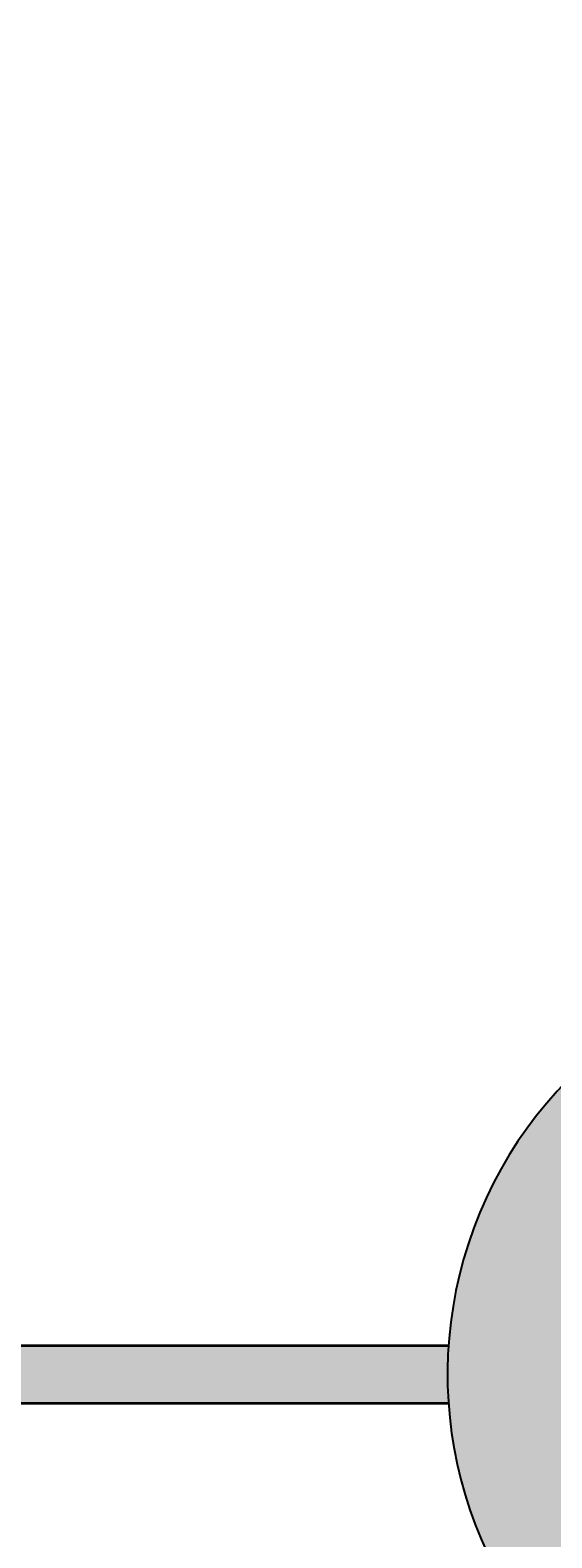
# Model space of a CAD drawing. Units: millimetres. Extents: x -22994 to 29398, y -19990 to 20176.
# Tile 11 of 135: x 32 to 41, y 26 to 52. Entities that reach past the tile are written whole.
import ezdxf
from ezdxf import colors
from ezdxf.entities.mleader import LeaderData, LeaderLine
from ezdxf.math import Vec2, Vec3

# ---------------------------------------------------------------- set-up
doc = ezdxf.new("R2010")
doc.units = ezdxf.units.MM
doc.header["$MEASUREMENT"] = 0
for name, color, linetype, lineweight in [('M-ANNO-TEXT', 7, 'Continuous', 25), ('M-DIMS', 2, 'Continuous', 18), ('M-EQPM', 7, 'Continuous', 25), ('M-EQPM-PATT', 7, 'Continuous', 18), ('M-PIPE', 7, 'Continuous', 35)]:
    doc.layers.add(name, color=color, linetype=linetype, lineweight=lineweight)
doc.styles.get("Standard").update_dxf_attribs({"font": 'arial.ttf'})
doc.dimstyles.get("Standard").update_dxf_attribs({"dimtxt": 0.18, "dimasz": 10000, "dimexe": 0.18, "dimexo": 0.0625, "dimgap": 0.09, "dimtad": 0, "dimtih": 1, "dimtoh": 1, "dimdec": 0, "dimzin": 0, "dimdsep": 46, "dimtxsty": 'Standard', "dimcen": 0.09, "dimadec": 0, "dimazin": 0, "dimtfac": 1, "dimtdec": 0, "dimtofl": 0, "dimtmove": 0, "dimatfit": 3, "dimfxl": 1, "dimtolj": 1, "dimtzin": 0, "dimlwd": 30, "dimarcsym": 0})

# ---------------------------------------------------------------- blocks, each defined once
blk = doc.blocks.new('*D2')
at = {"layer": 'Defpoints', "color": 0, "transparency": 16777216}
for p in [(6.677, 10.271), (290.852, 10.271), (290.852, -5.079)]:
    blk.add_point(p, dxfattribs=at)
at = {"layer": 'M-DIMS', "color": 0, "lineweight": -2, "transparency": 16777216}
for p, q in [((6.677, 10.209), (6.677, -5.259)), ((290.852, 10.209), (290.852, -5.259))]:
    blk.add_line(p, q, dxfattribs=at)
at = {"layer": 'M-DIMS', "color": 0, "lineweight": 30, "transparency": 16777216}
for p, q in [((-9993.323, -5.079), (-19993.323, -5.079)), ((10290.852, -5.079), (20290.852, -5.079))]:
    blk.add_line(p, q, dxfattribs=at)
at = {"layer": 'M-DIMS', "color": 0, "transparency": 16777216}
for points in [[(-9993.323, 1661.588), (-9993.323, -1671.745), (6.677, -5.079)], [(10290.852, 1661.588), (10290.852, -1671.745), (290.852, -5.079)]]:
    blk.add_solid(points, dxfattribs=at)
at = {"layer": 'M-DIMS', "color": 0, "transparency": 16777216, "insert": (148.765, -5.079), "char_height": 0.18, "attachment_point": 5}
blk.add_mtext('\\A1;284.2', dxfattribs=at)
blk = doc.blocks.new('*D3')
at = {"layer": 'Defpoints', "color": 0, "transparency": 16777216}
for p in [(110.265, 204.165), (110.265, 176.366), (95.833, 127.967)]:
    blk.add_point(p, dxfattribs=at)
at = {"layer": 'M-DIMS', "color": 0, "lineweight": -2, "transparency": 16777216}
for p, q in [((95.833, 128.03), (95.833, 204.345)), ((110.265, 176.429), (110.265, 204.345))]:
    blk.add_line(p, q, dxfattribs=at)
at = {"layer": 'M-DIMS', "color": 0, "lineweight": 30, "transparency": 16777216}
for p, q in [((-9904.167, 204.165), (-19904.167, 204.165)), ((10110.265, 204.165), (20110.265, 204.165))]:
    blk.add_line(p, q, dxfattribs=at)
at = {"layer": 'M-DIMS', "color": 0, "transparency": 16777216}
for points in [[(-9904.167, 1870.832), (-9904.167, -1462.501), (95.833, 204.165)], [(10110.265, 1870.832), (10110.265, -1462.501), (110.265, 204.165)]]:
    blk.add_solid(points, dxfattribs=at)
at = {"layer": 'M-DIMS', "color": 0, "transparency": 16777216, "insert": (103.049, 204.165), "char_height": 0.18, "attachment_point": 5}
blk.add_mtext('\\A1;14.432', dxfattribs=at)
blk = doc.blocks.new('*D4')
at = {"layer": 'Defpoints', "color": 0, "transparency": 16777216}
for p in [(116.265, 204.165), (110.265, 176.366), (116.265, 176.366)]:
    blk.add_point(p, dxfattribs=at)
at = {"layer": 'M-DIMS', "color": 0, "lineweight": -2, "transparency": 16777216}
for p, q in [((110.265, 176.429), (110.265, 204.345)), ((116.265, 176.429), (116.265, 204.345))]:
    blk.add_line(p, q, dxfattribs=at)
at = {"layer": 'M-DIMS', "color": 0, "lineweight": 30, "transparency": 16777216}
for p, q in [((-9889.735, 204.165), (-19889.735, 204.165)), ((10116.265, 204.165), (20116.265, 204.165))]:
    blk.add_line(p, q, dxfattribs=at)
at = {"layer": 'M-DIMS', "color": 0, "transparency": 16777216}
for points in [[(-9889.735, 1870.832), (-9889.735, -1462.501), (110.265, 204.165)], [(10116.265, 1870.832), (10116.265, -1462.501), (116.265, 204.165)]]:
    blk.add_solid(points, dxfattribs=at)
at = {"layer": 'M-DIMS', "color": 0, "transparency": 16777216, "insert": (113.265, 204.165), "char_height": 0.18, "attachment_point": 5}
blk.add_mtext('\\A1;6', dxfattribs=at)
blk = doc.blocks.new('*D5')
at = {"layer": 'Defpoints', "color": 0, "transparency": 16777216}
for p in [(181.265, 204.165), (116.265, 176.366), (181.265, 176.366)]:
    blk.add_point(p, dxfattribs=at)
at = {"layer": 'M-DIMS', "color": 0, "lineweight": -2, "transparency": 16777216}
for p, q in [((116.265, 176.429), (116.265, 204.345)), ((181.265, 176.429), (181.265, 204.345))]:
    blk.add_line(p, q, dxfattribs=at)
at = {"layer": 'M-DIMS', "color": 0, "lineweight": 30, "transparency": 16777216}
for p, q in [((-9883.735, 204.165), (-19883.735, 204.165)), ((10181.265, 204.165), (20181.265, 204.165))]:
    blk.add_line(p, q, dxfattribs=at)
at = {"layer": 'M-DIMS', "color": 0, "transparency": 16777216}
for points in [[(-9883.735, 1870.832), (-9883.735, -1462.501), (116.265, 204.165)], [(10181.265, 1870.832), (10181.265, -1462.501), (181.265, 204.165)]]:
    blk.add_solid(points, dxfattribs=at)
at = {"layer": 'M-DIMS', "color": 0, "transparency": 16777216, "insert": (148.765, 204.165), "char_height": 0.18, "attachment_point": 5}
blk.add_mtext('\\A1;65', dxfattribs=at)
blk = doc.blocks.new('*D6')
at = {"layer": 'Defpoints', "color": 0, "transparency": 16777216}
for p in [(187.265, 204.165), (181.265, 176.366), (187.265, 176.366)]:
    blk.add_point(p, dxfattribs=at)
at = {"layer": 'M-DIMS', "color": 0, "lineweight": -2, "transparency": 16777216}
for p, q in [((181.265, 176.429), (181.265, 204.345)), ((187.265, 176.429), (187.265, 204.345))]:
    blk.add_line(p, q, dxfattribs=at)
at = {"layer": 'M-DIMS', "color": 0, "lineweight": 30, "transparency": 16777216}
for p, q in [((-9818.735, 204.165), (-19818.735, 204.165)), ((10187.265, 204.165), (20187.265, 204.165))]:
    blk.add_line(p, q, dxfattribs=at)
at = {"layer": 'M-DIMS', "color": 0, "transparency": 16777216}
for points in [[(-9818.735, 1870.832), (-9818.735, -1462.501), (181.265, 204.165)], [(10187.265, 1870.832), (10187.265, -1462.501), (187.265, 204.165)]]:
    blk.add_solid(points, dxfattribs=at)
at = {"layer": 'M-DIMS', "color": 0, "transparency": 16777216, "insert": (184.265, 204.165), "char_height": 0.18, "attachment_point": 5}
blk.add_mtext('\\A1;6', dxfattribs=at)
blk = doc.blocks.new('*D7')
at = {"layer": 'Defpoints', "color": 0, "transparency": 16777216}
for p in [(201.697, 204.165), (187.265, 176.366), (201.697, 127.967)]:
    blk.add_point(p, dxfattribs=at)
at = {"layer": 'M-DIMS', "color": 0, "lineweight": -2, "transparency": 16777216}
for p, q in [((187.265, 176.429), (187.265, 204.345)), ((201.697, 128.03), (201.697, 204.345))]:
    blk.add_line(p, q, dxfattribs=at)
at = {"layer": 'M-DIMS', "color": 0, "lineweight": 30, "transparency": 16777216}
for p, q in [((-9812.735, 204.165), (-19812.735, 204.165)), ((10201.697, 204.165), (20201.697, 204.165))]:
    blk.add_line(p, q, dxfattribs=at)
at = {"layer": 'M-DIMS', "color": 0, "transparency": 16777216}
for points in [[(-9812.735, 1870.832), (-9812.735, -1462.501), (187.265, 204.165)], [(10201.697, 1870.832), (10201.697, -1462.501), (201.697, 204.165)]]:
    blk.add_solid(points, dxfattribs=at)
at = {"layer": 'M-DIMS', "color": 0, "transparency": 16777216, "insert": (194.481, 204.165), "char_height": 0.18, "attachment_point": 5}
blk.add_mtext('\\A1;14.432', dxfattribs=at)
blk = doc.blocks.new('*D8')
at = {"layer": 'Defpoints', "color": 0, "transparency": 16777216}
for p in [(227.648, 204.165), (227.648, 146.73), (201.697, 127.967)]:
    blk.add_point(p, dxfattribs=at)
at = {"layer": 'M-DIMS', "color": 0, "lineweight": -2, "transparency": 16777216}
for p, q in [((201.697, 128.03), (201.697, 204.345)), ((227.648, 146.792), (227.648, 204.345))]:
    blk.add_line(p, q, dxfattribs=at)
at = {"layer": 'M-DIMS', "color": 0, "lineweight": 30, "transparency": 16777216}
for p, q in [((-9798.303, 204.165), (-19798.303, 204.165)), ((10227.648, 204.165), (20227.648, 204.165))]:
    blk.add_line(p, q, dxfattribs=at)
at = {"layer": 'M-DIMS', "color": 0, "transparency": 16777216}
for points in [[(-9798.303, 1870.832), (-9798.303, -1462.501), (201.697, 204.165)], [(10227.648, 1870.832), (10227.648, -1462.501), (227.648, 204.165)]]:
    blk.add_solid(points, dxfattribs=at)
at = {"layer": 'M-DIMS', "color": 0, "transparency": 16777216, "insert": (214.673, 204.165), "char_height": 0.18, "attachment_point": 5}
blk.add_mtext('\\A1;25.95', dxfattribs=at)
blk = doc.blocks.new('*D9')
at = {"layer": 'Defpoints', "color": 0, "transparency": 16777216}
for p in [(187.265, 176.366), (306.202, 176.366), (290.852, 10.271)]:
    blk.add_point(p, dxfattribs=at)
at = {"layer": 'M-DIMS', "color": 0, "lineweight": 30, "transparency": 16777216}
for p, q in [((306.202, 10176.366), (306.202, 20176.366)), ((306.202, -9989.729), (306.202, -19989.729))]:
    blk.add_line(p, q, dxfattribs=at)
at = {"layer": 'M-DIMS', "color": 0, "lineweight": -2, "transparency": 16777216}
for p, q in [((187.327, 176.366), (306.382, 176.366)), ((290.915, 10.271), (306.382, 10.271))]:
    blk.add_line(p, q, dxfattribs=at)
at = {"layer": 'M-DIMS', "color": 0, "transparency": 16777216}
for points in [[(-1360.465, 10176.366), (1972.869, 10176.366), (306.202, 176.366)], [(-1360.465, -9989.729), (1972.869, -9989.729), (306.202, 10.271)]]:
    blk.add_solid(points, dxfattribs=at)
at = {"layer": 'M-DIMS', "color": 0, "transparency": 16777216, "insert": (306.202, 93.319), "char_height": 0.18, "attachment_point": 5}
blk.add_mtext('\\A1;166.1', dxfattribs=at)
blk = doc.blocks.new('*D10')
at = {"layer": 'Defpoints', "color": 0, "transparency": 16777216}
for p in [(125.65, 136.071), (133.346, 136.071), (133.346, -5.079)]:
    blk.add_point(p, dxfattribs=at)
at = {"layer": 'M-DIMS', "color": 0, "lineweight": -2, "transparency": 16777216}
for p, q in [((125.65, 136.009), (125.65, -5.259)), ((133.346, 136.009), (133.346, -5.259))]:
    blk.add_line(p, q, dxfattribs=at)
at = {"layer": 'M-DIMS', "color": 0, "lineweight": 30, "transparency": 16777216}
for p, q in [((-9874.35, -5.079), (-19874.35, -5.079)), ((10133.346, -5.079), (20133.346, -5.079))]:
    blk.add_line(p, q, dxfattribs=at)
at = {"layer": 'M-DIMS', "color": 0, "transparency": 16777216}
for points in [[(-9874.35, 1661.588), (-9874.35, -1671.745), (125.65, -5.079)], [(10133.346, 1661.588), (10133.346, -1671.745), (133.346, -5.079)]]:
    blk.add_solid(points, dxfattribs=at)
at = {"layer": 'M-DIMS', "color": 0, "transparency": 16777216, "insert": (129.498, -5.079), "char_height": 0.18, "attachment_point": 5}
blk.add_mtext('\\A1;7.696', dxfattribs=at)
blk = doc.blocks.new('*D11')
at = {"layer": 'Defpoints', "color": 0, "transparency": 16777216}
for p in [(133.346, 136.071), (135.65, 136.071), (135.65, -5.079)]:
    blk.add_point(p, dxfattribs=at)
at = {"layer": 'M-DIMS', "color": 0, "lineweight": -2, "transparency": 16777216}
for p, q in [((133.346, 136.009), (133.346, -5.259)), ((135.65, 136.009), (135.65, -5.259))]:
    blk.add_line(p, q, dxfattribs=at)
at = {"layer": 'M-DIMS', "color": 0, "lineweight": 30, "transparency": 16777216}
for p, q in [((-9866.654, -5.079), (-19866.654, -5.079)), ((10135.65, -5.079), (20135.65, -5.079))]:
    blk.add_line(p, q, dxfattribs=at)
at = {"layer": 'M-DIMS', "color": 0, "transparency": 16777216}
for points in [[(-9866.654, 1661.588), (-9866.654, -1671.745), (133.346, -5.079)], [(10135.65, 1661.588), (10135.65, -1671.745), (135.65, -5.079)]]:
    blk.add_solid(points, dxfattribs=at)
at = {"layer": 'M-DIMS', "color": 0, "transparency": 16777216, "insert": (134.498, -5.079), "char_height": 0.18, "attachment_point": 5}
blk.add_mtext('\\A1;2.304', dxfattribs=at)
blk = doc.blocks.new('*D12')
at = {"layer": 'Defpoints', "color": 0, "transparency": 16777216}
for p in [(135.65, 136.071), (145.65, 136.071), (145.65, -5.079)]:
    blk.add_point(p, dxfattribs=at)
at = {"layer": 'M-DIMS', "color": 0, "lineweight": -2, "transparency": 16777216}
for p, q in [((135.65, 136.009), (135.65, -5.259)), ((145.65, 136.009), (145.65, -5.259))]:
    blk.add_line(p, q, dxfattribs=at)
at = {"layer": 'M-DIMS', "color": 0, "lineweight": 30, "transparency": 16777216}
for p, q in [((-9864.35, -5.079), (-19864.35, -5.079)), ((10145.65, -5.079), (20145.65, -5.079))]:
    blk.add_line(p, q, dxfattribs=at)
at = {"layer": 'M-DIMS', "color": 0, "transparency": 16777216}
for points in [[(-9864.35, 1661.588), (-9864.35, -1671.745), (135.65, -5.079)], [(10145.65, 1661.588), (10145.65, -1671.745), (145.65, -5.079)]]:
    blk.add_solid(points, dxfattribs=at)
at = {"layer": 'M-DIMS', "color": 0, "transparency": 16777216, "insert": (140.65, -5.079), "char_height": 0.18, "attachment_point": 5}
blk.add_mtext('\\A1;10', dxfattribs=at)
blk = doc.blocks.new('*D13')
at = {"layer": 'Defpoints', "color": 0, "transparency": 16777216}
for p in [(145.65, 136.071), (155.65, 136.071), (155.65, -5.079)]:
    blk.add_point(p, dxfattribs=at)
at = {"layer": 'M-DIMS', "color": 0, "lineweight": -2, "transparency": 16777216}
for p, q in [((145.65, 136.009), (145.65, -5.259)), ((155.65, 136.009), (155.65, -5.259))]:
    blk.add_line(p, q, dxfattribs=at)
at = {"layer": 'M-DIMS', "color": 0, "lineweight": 30, "transparency": 16777216}
for p, q in [((-9854.35, -5.079), (-19854.35, -5.079)), ((10155.65, -5.079), (20155.65, -5.079))]:
    blk.add_line(p, q, dxfattribs=at)
at = {"layer": 'M-DIMS', "color": 0, "transparency": 16777216}
for points in [[(-9854.35, 1661.588), (-9854.35, -1671.745), (145.65, -5.079)], [(10155.65, 1661.588), (10155.65, -1671.745), (155.65, -5.079)]]:
    blk.add_solid(points, dxfattribs=at)
at = {"layer": 'M-DIMS', "color": 0, "transparency": 16777216, "insert": (150.65, -5.079), "char_height": 0.18, "attachment_point": 5}
blk.add_mtext('\\A1;10', dxfattribs=at)
blk = doc.blocks.new('*D14')
at = {"layer": 'Defpoints', "color": 0, "transparency": 16777216}
for p in [(155.65, 136.071), (165.65, 136.071), (165.65, -5.079)]:
    blk.add_point(p, dxfattribs=at)
at = {"layer": 'M-DIMS', "color": 0, "lineweight": -2, "transparency": 16777216}
for p, q in [((155.65, 136.009), (155.65, -5.259)), ((165.65, 136.009), (165.65, -5.259))]:
    blk.add_line(p, q, dxfattribs=at)
at = {"layer": 'M-DIMS', "color": 0, "lineweight": 30, "transparency": 16777216}
for p, q in [((-9844.35, -5.079), (-19844.35, -5.079)), ((10165.65, -5.079), (20165.65, -5.079))]:
    blk.add_line(p, q, dxfattribs=at)
at = {"layer": 'M-DIMS', "color": 0, "transparency": 16777216}
for points in [[(-9844.35, 1661.588), (-9844.35, -1671.745), (155.65, -5.079)], [(10165.65, 1661.588), (10165.65, -1671.745), (165.65, -5.079)]]:
    blk.add_solid(points, dxfattribs=at)
at = {"layer": 'M-DIMS', "color": 0, "transparency": 16777216, "insert": (160.65, -5.079), "char_height": 0.18, "attachment_point": 5}
blk.add_mtext('\\A1;10', dxfattribs=at)
blk = doc.blocks.new('*D15')
at = {"layer": 'Defpoints', "color": 0, "transparency": 16777216}
for p in [(173.346, 154.788), (173.346, 136.071), (306.202, 136.071)]:
    blk.add_point(p, dxfattribs=at)
at = {"layer": 'M-DIMS', "color": 0, "lineweight": 30, "transparency": 16777216}
for p, q in [((306.202, 10154.788), (306.202, 20154.788)), ((306.202, -9863.929), (306.202, -19863.929))]:
    blk.add_line(p, q, dxfattribs=at)
at = {"layer": 'M-DIMS', "color": 0, "lineweight": -2, "transparency": 16777216}
for p, q in [((173.408, 154.788), (306.382, 154.788)), ((173.408, 136.071), (306.382, 136.071))]:
    blk.add_line(p, q, dxfattribs=at)
at = {"layer": 'M-DIMS', "color": 0, "transparency": 16777216}
for points in [[(-1360.465, 10154.788), (1972.869, 10154.788), (306.202, 154.788)], [(-1360.465, -9863.929), (1972.869, -9863.929), (306.202, 136.071)]]:
    blk.add_solid(points, dxfattribs=at)
at = {"layer": 'M-DIMS', "color": 0, "transparency": 16777216, "insert": (306.202, 145.43), "char_height": 0.18, "attachment_point": 5}
blk.add_mtext('\\A1;18.717', dxfattribs=at)
blk = doc.blocks.new('*D16')
at = {"layer": 'Defpoints', "color": 0, "transparency": 16777216}
for p in [(120.17, 204.165), (110.466, 48.035), (120.17, 48.035)]:
    blk.add_point(p, dxfattribs=at)
at = {"layer": 'M-DIMS', "color": 0, "lineweight": -2, "transparency": 16777216}
for p, q in [((110.466, 48.097), (110.466, 204.345)), ((120.17, 48.097), (120.17, 204.345))]:
    blk.add_line(p, q, dxfattribs=at)
at = {"layer": 'M-DIMS', "color": 0, "lineweight": 30, "transparency": 16777216}
for p, q in [((-9889.534, 204.165), (-19889.534, 204.165)), ((10120.17, 204.165), (20120.17, 204.165))]:
    blk.add_line(p, q, dxfattribs=at)
at = {"layer": 'M-DIMS', "color": 0, "transparency": 16777216}
for points in [[(-9889.534, 1870.832), (-9889.534, -1462.501), (110.466, 204.165)], [(10120.17, 1870.832), (10120.17, -1462.501), (120.17, 204.165)]]:
    blk.add_solid(points, dxfattribs=at)
at = {"layer": 'M-DIMS', "color": 0, "transparency": 16777216, "insert": (115.318, 204.165), "char_height": 0.18, "attachment_point": 5}
blk.add_mtext('\\A1;9.704', dxfattribs=at)
blk = doc.blocks.new('*D17')
at = {"layer": 'Defpoints', "color": 0, "transparency": 16777216}
for p in [(126.17, 204.165), (120.17, 48.035), (126.17, 48.035)]:
    blk.add_point(p, dxfattribs=at)
at = {"layer": 'M-DIMS', "color": 0, "lineweight": -2, "transparency": 16777216}
for p, q in [((120.17, 48.097), (120.17, 204.345)), ((126.17, 48.097), (126.17, 204.345))]:
    blk.add_line(p, q, dxfattribs=at)
at = {"layer": 'M-DIMS', "color": 0, "lineweight": 30, "transparency": 16777216}
for p, q in [((-9879.83, 204.165), (-19879.83, 204.165)), ((10126.17, 204.165), (20126.17, 204.165))]:
    blk.add_line(p, q, dxfattribs=at)
at = {"layer": 'M-DIMS', "color": 0, "transparency": 16777216}
for points in [[(-9879.83, 1870.832), (-9879.83, -1462.501), (120.17, 204.165)], [(10126.17, 1870.832), (10126.17, -1462.501), (126.17, 204.165)]]:
    blk.add_solid(points, dxfattribs=at)
at = {"layer": 'M-DIMS', "color": 0, "transparency": 16777216, "insert": (123.17, 204.165), "char_height": 0.18, "attachment_point": 5}
blk.add_mtext('\\A1;6', dxfattribs=at)
blk = doc.blocks.new('*D18')
at = {"layer": 'Defpoints', "color": 0, "transparency": 16777216}
for p in [(132.17, 204.165), (126.17, 48.035), (132.17, 48.035)]:
    blk.add_point(p, dxfattribs=at)
at = {"layer": 'M-DIMS', "color": 0, "lineweight": -2, "transparency": 16777216}
for p, q in [((126.17, 48.097), (126.17, 204.345)), ((132.17, 48.097), (132.17, 204.345))]:
    blk.add_line(p, q, dxfattribs=at)
at = {"layer": 'M-DIMS', "color": 0, "lineweight": 30, "transparency": 16777216}
for p, q in [((-9873.83, 204.165), (-19873.83, 204.165)), ((10132.17, 204.165), (20132.17, 204.165))]:
    blk.add_line(p, q, dxfattribs=at)
at = {"layer": 'M-DIMS', "color": 0, "transparency": 16777216}
for points in [[(-9873.83, 1870.832), (-9873.83, -1462.501), (126.17, 204.165)], [(10132.17, 1870.832), (10132.17, -1462.501), (132.17, 204.165)]]:
    blk.add_solid(points, dxfattribs=at)
at = {"layer": 'M-DIMS', "color": 0, "transparency": 16777216, "insert": (129.17, 204.165), "char_height": 0.18, "attachment_point": 5}
blk.add_mtext('\\A1;6', dxfattribs=at)
blk = doc.blocks.new('*D19')
at = {"layer": 'Defpoints', "color": 0, "transparency": 16777216}
for p in [(138.17, 204.165), (132.17, 48.035), (138.17, 48.035)]:
    blk.add_point(p, dxfattribs=at)
at = {"layer": 'M-DIMS', "color": 0, "lineweight": -2, "transparency": 16777216}
for p, q in [((132.17, 48.097), (132.17, 204.345)), ((138.17, 48.097), (138.17, 204.345))]:
    blk.add_line(p, q, dxfattribs=at)
at = {"layer": 'M-DIMS', "color": 0, "lineweight": 30, "transparency": 16777216}
for p, q in [((-9867.83, 204.165), (-19867.83, 204.165)), ((10138.17, 204.165), (20138.17, 204.165))]:
    blk.add_line(p, q, dxfattribs=at)
at = {"layer": 'M-DIMS', "color": 0, "transparency": 16777216}
for points in [[(-9867.83, 1870.832), (-9867.83, -1462.501), (132.17, 204.165)], [(10138.17, 1870.832), (10138.17, -1462.501), (138.17, 204.165)]]:
    blk.add_solid(points, dxfattribs=at)
at = {"layer": 'M-DIMS', "color": 0, "transparency": 16777216, "insert": (135.17, 204.165), "char_height": 0.18, "attachment_point": 5}
blk.add_mtext('\\A1;6', dxfattribs=at)
blk = doc.blocks.new('*D20')
at = {"layer": 'Defpoints', "color": 0, "transparency": 16777216}
for p in [(144.17, 204.165), (138.17, 48.035), (144.17, 48.035)]:
    blk.add_point(p, dxfattribs=at)
at = {"layer": 'M-DIMS', "color": 0, "lineweight": -2, "transparency": 16777216}
for p, q in [((138.17, 48.097), (138.17, 204.345)), ((144.17, 48.097), (144.17, 204.345))]:
    blk.add_line(p, q, dxfattribs=at)
at = {"layer": 'M-DIMS', "color": 0, "lineweight": 30, "transparency": 16777216}
for p, q in [((-9861.83, 204.165), (-19861.83, 204.165)), ((10144.17, 204.165), (20144.17, 204.165))]:
    blk.add_line(p, q, dxfattribs=at)
at = {"layer": 'M-DIMS', "color": 0, "transparency": 16777216}
for points in [[(-9861.83, 1870.832), (-9861.83, -1462.501), (138.17, 204.165)], [(10144.17, 1870.832), (10144.17, -1462.501), (144.17, 204.165)]]:
    blk.add_solid(points, dxfattribs=at)
at = {"layer": 'M-DIMS', "color": 0, "transparency": 16777216, "insert": (141.17, 204.165), "char_height": 0.18, "attachment_point": 5}
blk.add_mtext('\\A1;6', dxfattribs=at)
blk = doc.blocks.new('*D21')
at = {"layer": 'Defpoints', "color": 0, "transparency": 16777216}
for p in [(149.116, 204.165), (144.17, 48.035), (149.116, 48.035)]:
    blk.add_point(p, dxfattribs=at)
at = {"layer": 'M-DIMS', "color": 0, "lineweight": -2, "transparency": 16777216}
for p, q in [((144.17, 48.097), (144.17, 204.345)), ((149.116, 48.097), (149.116, 204.345))]:
    blk.add_line(p, q, dxfattribs=at)
at = {"layer": 'M-DIMS', "color": 0, "lineweight": 30, "transparency": 16777216}
for p, q in [((-9855.83, 204.165), (-19855.83, 204.165)), ((10149.116, 204.165), (20149.116, 204.165))]:
    blk.add_line(p, q, dxfattribs=at)
at = {"layer": 'M-DIMS', "color": 0, "transparency": 16777216}
for points in [[(-9855.83, 1870.832), (-9855.83, -1462.501), (144.17, 204.165)], [(10149.116, 1870.832), (10149.116, -1462.501), (149.116, 204.165)]]:
    blk.add_solid(points, dxfattribs=at)
at = {"layer": 'M-DIMS', "color": 0, "transparency": 16777216, "insert": (146.643, 204.165), "char_height": 0.18, "attachment_point": 5}
blk.add_mtext('\\A1;4.945', dxfattribs=at)
blk = doc.blocks.new('*D22')
at = {"layer": 'Defpoints', "color": 0, "transparency": 16777216}
for p in [(149.116, 30.99), (155.116, 30.99), (155.116, -5.079)]:
    blk.add_point(p, dxfattribs=at)
at = {"layer": 'M-DIMS', "color": 0, "lineweight": -2, "transparency": 16777216}
for p, q in [((149.116, 30.927), (149.116, -5.259)), ((155.116, 30.927), (155.116, -5.259))]:
    blk.add_line(p, q, dxfattribs=at)
at = {"layer": 'M-DIMS', "color": 0, "lineweight": 30, "transparency": 16777216}
for p, q in [((-9850.884, -5.079), (-19850.884, -5.079)), ((10155.116, -5.079), (20155.116, -5.079))]:
    blk.add_line(p, q, dxfattribs=at)
at = {"layer": 'M-DIMS', "color": 0, "transparency": 16777216}
for points in [[(-9850.884, 1661.588), (-9850.884, -1671.745), (149.116, -5.079)], [(10155.116, 1661.588), (10155.116, -1671.745), (155.116, -5.079)]]:
    blk.add_solid(points, dxfattribs=at)
at = {"layer": 'M-DIMS', "color": 0, "transparency": 16777216, "insert": (152.116, -5.079), "char_height": 0.18, "attachment_point": 5}
blk.add_mtext('\\A1;6', dxfattribs=at)
blk = doc.blocks.new('*D23')
at = {"layer": 'Defpoints', "color": 0, "transparency": 16777216}
for p in [(155.116, 30.99), (161.116, 30.99), (161.116, -5.079)]:
    blk.add_point(p, dxfattribs=at)
at = {"layer": 'M-DIMS', "color": 0, "lineweight": -2, "transparency": 16777216}
for p, q in [((155.116, 30.927), (155.116, -5.259)), ((161.116, 30.927), (161.116, -5.259))]:
    blk.add_line(p, q, dxfattribs=at)
at = {"layer": 'M-DIMS', "color": 0, "lineweight": 30, "transparency": 16777216}
for p, q in [((-9844.884, -5.079), (-19844.884, -5.079)), ((10161.116, -5.079), (20161.116, -5.079))]:
    blk.add_line(p, q, dxfattribs=at)
at = {"layer": 'M-DIMS', "color": 0, "transparency": 16777216}
for points in [[(-9844.884, 1661.588), (-9844.884, -1671.745), (155.116, -5.079)], [(10161.116, 1661.588), (10161.116, -1671.745), (161.116, -5.079)]]:
    blk.add_solid(points, dxfattribs=at)
at = {"layer": 'M-DIMS', "color": 0, "transparency": 16777216, "insert": (158.116, -5.079), "char_height": 0.18, "attachment_point": 5}
blk.add_mtext('\\A1;6', dxfattribs=at)
blk = doc.blocks.new('*D24')
at = {"layer": 'Defpoints', "color": 0, "transparency": 16777216}
for p in [(161.116, 30.99), (166.439, 30.99), (166.439, -5.079)]:
    blk.add_point(p, dxfattribs=at)
at = {"layer": 'M-DIMS', "color": 0, "lineweight": -2, "transparency": 16777216}
for p, q in [((161.116, 30.927), (161.116, -5.259)), ((166.439, 30.927), (166.439, -5.259))]:
    blk.add_line(p, q, dxfattribs=at)
at = {"layer": 'M-DIMS', "color": 0, "lineweight": 30, "transparency": 16777216}
for p, q in [((-9838.884, -5.079), (-19838.884, -5.079)), ((10166.439, -5.079), (20166.439, -5.079))]:
    blk.add_line(p, q, dxfattribs=at)
at = {"layer": 'M-DIMS', "color": 0, "transparency": 16777216}
for points in [[(-9838.884, 1661.588), (-9838.884, -1671.745), (161.116, -5.079)], [(10166.439, 1661.588), (10166.439, -1671.745), (166.439, -5.079)]]:
    blk.add_solid(points, dxfattribs=at)
at = {"layer": 'M-DIMS', "color": 0, "transparency": 16777216, "insert": (163.777, -5.079), "char_height": 0.18, "attachment_point": 5}
blk.add_mtext('\\A1;5.323', dxfattribs=at)
blk = doc.blocks.new('*D25')
at = {"layer": 'Defpoints', "color": 0, "transparency": 16777216}
for p in [(166.439, 30.99), (172.439, 30.99), (172.439, -5.079)]:
    blk.add_point(p, dxfattribs=at)
at = {"layer": 'M-DIMS', "color": 0, "lineweight": -2, "transparency": 16777216}
for p, q in [((166.439, 30.927), (166.439, -5.259)), ((172.439, 30.927), (172.439, -5.259))]:
    blk.add_line(p, q, dxfattribs=at)
at = {"layer": 'M-DIMS', "color": 0, "lineweight": 30, "transparency": 16777216}
for p, q in [((-9833.561, -5.079), (-19833.561, -5.079)), ((10172.439, -5.079), (20172.439, -5.079))]:
    blk.add_line(p, q, dxfattribs=at)
at = {"layer": 'M-DIMS', "color": 0, "transparency": 16777216}
for points in [[(-9833.561, 1661.588), (-9833.561, -1671.745), (166.439, -5.079)], [(10172.439, 1661.588), (10172.439, -1671.745), (172.439, -5.079)]]:
    blk.add_solid(points, dxfattribs=at)
at = {"layer": 'M-DIMS', "color": 0, "transparency": 16777216, "insert": (169.439, -5.079), "char_height": 0.18, "attachment_point": 5}
blk.add_mtext('\\A1;6', dxfattribs=at)
blk = doc.blocks.new('*D26')
at = {"layer": 'Defpoints', "color": 0, "transparency": 16777216}
for p in [(172.439, 30.99), (178.439, 30.99), (178.439, -5.079)]:
    blk.add_point(p, dxfattribs=at)
at = {"layer": 'M-DIMS', "color": 0, "lineweight": -2, "transparency": 16777216}
for p, q in [((172.439, 30.927), (172.439, -5.259)), ((178.439, 30.927), (178.439, -5.259))]:
    blk.add_line(p, q, dxfattribs=at)
at = {"layer": 'M-DIMS', "color": 0, "lineweight": 30, "transparency": 16777216}
for p, q in [((-9827.561, -5.079), (-19827.561, -5.079)), ((10178.439, -5.079), (20178.439, -5.079))]:
    blk.add_line(p, q, dxfattribs=at)
at = {"layer": 'M-DIMS', "color": 0, "transparency": 16777216}
for points in [[(-9827.561, 1661.588), (-9827.561, -1671.745), (172.439, -5.079)], [(10178.439, 1661.588), (10178.439, -1671.745), (178.439, -5.079)]]:
    blk.add_solid(points, dxfattribs=at)
at = {"layer": 'M-DIMS', "color": 0, "transparency": 16777216, "insert": (175.439, -5.079), "char_height": 0.18, "attachment_point": 5}
blk.add_mtext('\\A1;6', dxfattribs=at)
blk = doc.blocks.new('*D27')
at = {"layer": 'Defpoints', "color": 0, "transparency": 16777216}
for p in [(178.439, 30.99), (188.117, 30.99), (188.117, -5.079)]:
    blk.add_point(p, dxfattribs=at)
at = {"layer": 'M-DIMS', "color": 0, "lineweight": -2, "transparency": 16777216}
for p, q in [((178.439, 30.927), (178.439, -5.259)), ((188.117, 30.927), (188.117, -5.259))]:
    blk.add_line(p, q, dxfattribs=at)
at = {"layer": 'M-DIMS', "color": 0, "lineweight": 30, "transparency": 16777216}
for p, q in [((-9821.561, -5.079), (-19821.561, -5.079)), ((10188.117, -5.079), (20188.117, -5.079))]:
    blk.add_line(p, q, dxfattribs=at)
at = {"layer": 'M-DIMS', "color": 0, "transparency": 16777216}
for points in [[(-9821.561, 1661.588), (-9821.561, -1671.745), (178.439, -5.079)], [(10188.117, 1661.588), (10188.117, -1671.745), (188.117, -5.079)]]:
    blk.add_solid(points, dxfattribs=at)
at = {"layer": 'M-DIMS', "color": 0, "transparency": 16777216, "insert": (183.278, -5.079), "char_height": 0.18, "attachment_point": 5}
blk.add_mtext('\\A1;9.679', dxfattribs=at)
blk = doc.blocks.new('*D28')
at = {"layer": 'Defpoints', "color": 0, "transparency": 16777216}
for p in [(188.117, 48.035), (306.202, 48.035), (188.117, 30.99)]:
    blk.add_point(p, dxfattribs=at)
at = {"layer": 'M-DIMS', "color": 0, "lineweight": 30, "transparency": 16777216}
for p, q in [((306.202, 10048.035), (306.202, 20048.035)), ((306.202, -9969.01), (306.202, -19969.01))]:
    blk.add_line(p, q, dxfattribs=at)
at = {"layer": 'M-DIMS', "color": 0, "lineweight": -2, "transparency": 16777216}
for p, q in [((188.18, 48.035), (306.382, 48.035)), ((188.18, 30.99), (306.382, 30.99))]:
    blk.add_line(p, q, dxfattribs=at)
at = {"layer": 'M-DIMS', "color": 0, "transparency": 16777216}
for points in [[(-1360.465, 10048.035), (1972.869, 10048.035), (306.202, 48.035)], [(-1360.465, -9969.01), (1972.869, -9969.01), (306.202, 30.99)]]:
    blk.add_solid(points, dxfattribs=at)
at = {"layer": 'M-DIMS', "color": 0, "transparency": 16777216, "insert": (306.202, 39.512), "char_height": 0.18, "attachment_point": 5}
blk.add_mtext('\\A1;17.045', dxfattribs=at)
blk = doc.blocks.new('*D29')
at = {"layer": 'Defpoints', "color": 0, "transparency": 16777216}
for p in [(36.801, 80.045), (64.03, 80.045)]:
    blk.add_point(p, dxfattribs=at)
at = {"layer": 'M-DIMS', "color": 0, "lineweight": -2, "transparency": 16777216}
for p, q in [((50.415, 79.955), (50.415, 80.135)), ((50.325, 80.045), (50.505, 80.045))]:
    blk.add_line(p, q, dxfattribs=at)
at = {"layer": 'M-DIMS', "color": 0, "lineweight": 30, "transparency": 16777216}
blk.add_line((20064.03, 80.03), (10064.03, 80.038), dxfattribs=at)
at = {"layer": 'M-DIMS', "color": 0, "transparency": 16777216}
blk.add_solid([(10064.031, 1746.704), (10064.028, -1586.629), (64.03, 80.045)], dxfattribs=at)
at = {"layer": 'M-DIMS', "color": 0, "transparency": 16777216, "insert": (20064.521, 80.03), "char_height": 0.18, "attachment_point": 5}
blk.add_mtext('\\A1;∅27.23', dxfattribs=at)
blk = doc.blocks.new('*D32')
at = {"layer": 'Defpoints', "color": 0, "transparency": 16777216}
for p in [(57.164, 118.614), (52.413, 113.093)]:
    blk.add_point(p, dxfattribs=at)
at = {"layer": 'M-DIMS', "color": 0, "lineweight": -2, "transparency": 16777216}
for p, q in [((57.074, 118.614), (57.254, 118.614)), ((57.164, 118.524), (57.164, 118.704))]:
    blk.add_line(p, q, dxfattribs=at)
at = {"layer": 'M-DIMS', "color": 0, "lineweight": 30, "transparency": 16777216}
for p, q in [((-12992.534, -15047.031), (-6470.06, -7466.969)), ((-22992.534, -15047.031), (-12992.534, -15047.031))]:
    blk.add_line(p, q, dxfattribs=at)
at = {"layer": 'M-DIMS', "color": 0, "transparency": 16777216}
blk.add_solid([(-7733.404, -6379.89), (-5206.717, -8554.048), (52.413, 113.093)], dxfattribs=at)
at = {"layer": 'M-DIMS', "color": 0, "transparency": 16777216, "insert": (-22993.208, -15047.031), "char_height": 0.18, "attachment_point": 5}
blk.add_mtext('\\A1;2X R7.284', dxfattribs=at)
blk = doc.blocks.new('*D36')
at = {"layer": 'Defpoints', "color": 0, "transparency": 16777216}
for p in [(46.39, 31.303), (46.387, 26.593)]:
    blk.add_point(p, dxfattribs=at)
at = {"layer": 'M-DIMS', "color": 0, "lineweight": 30, "transparency": 16777216}
for p, q in [((57.15, 20031.301), (51.77, 10031.302)), ((10057.15, 20031.301), (57.15, 20031.301))]:
    blk.add_line(p, q, dxfattribs=at)
at = {"layer": 'M-DIMS', "color": 0, "lineweight": -2, "transparency": 16777216}
for p, q in [((46.389, 28.858), (46.389, 29.038)), ((46.299, 28.948), (46.479, 28.948))]:
    blk.add_line(p, q, dxfattribs=at)
at = {"layer": 'M-DIMS', "color": 0, "transparency": 16777216}
blk.add_solid([(-1614.896, 10032.199), (1718.436, 10030.405), (46.39, 31.303)], dxfattribs=at)
at = {"layer": 'M-DIMS', "color": 0, "transparency": 16777216, "insert": (10057.554, 20031.301), "char_height": 0.18, "attachment_point": 5}
blk.add_mtext('\\A1;∅4.71', dxfattribs=at)

msp = doc.modelspace()

# ---------------------------------------------------------------- hatches: boundary and pattern name
at = {"layer": 'M-EQPM-PATT'}
h = msp.add_hatch(color=256, dxfattribs=at)
h.set_gradient(color1=(242, 103, 34), color2=(242, 103, 34), tint=1, name='CYLINDER')
h.paths.add_polyline_path([(53.5912, 30.0354), (64.8905, 30.0354), (64.8905, 36.2325), (46.3887, 36.2325, 2.6954641)])
h.paths.add_polyline_path([(44.0337, 28.9485, -1), (48.7438, 28.9485, -1)], flags=16)
h.paths.add_polyline_path([(75.6657, 119.7012), (75.6657, 125.8983), (57.1639, 125.8983, 2.6954641), (64.3664, 119.7012)])
h.paths.add_polyline_path([(59.4936, 118.6143, -1), (54.8343, 118.6143, -1)], flags=16)
h = msp.add_hatch(color=256, dxfattribs=at)
h.set_gradient(color1=(16, 86, 137), color2=(39, 118, 187), tint=1, name='CYLINDER')
h.paths.add_polyline_path([(22.8402, 76.5922), (37.2457, 76.5922, -0.0188178), (37.0234, 77.5922), (21.8402, 77.5922, 0.4142136), (20.3402, 76.0922), (20.3402, 29.9485, 0.4142136), (21.8402, 28.4485), (39.1219, 28.4485, -0.0343621), (39.1219, 29.4485), (22.8402, 29.4485, -0.4142136), (21.3402, 30.9485), (21.3402, 75.0922, -0.4142136)])

# ---------------------------------------------------------------- linework, layer by layer
at = {"layer": 'M-EQPM'}
msp.add_arc((46.3887, 28.9485), 7.284, 90, 8.58187, dxfattribs=at)
at = {"layer": 'M-PIPE'}
for points in [[(37.0234, 77.5922), (21.8402, 77.5922, 0.4142136), (20.3402, 76.0922), (20.3402, 29.9485, 0.4142136), (21.8402, 28.4485), (39.1219, 28.4485)], [(37.2457, 76.5922), (22.8402, 76.5922, 0.4142136), (21.3402, 75.0922), (21.3402, 30.9485, 0.4142136), (22.8402, 29.4485), (39.1219, 29.4485)]]:
    msp.add_lwpolyline(points, format="xyb", dxfattribs=at)

# ---------------------------------------------------------------- dimensions: what is measured, and where the dimension line sits
at = {"layer": 'M-DIMS'}
for base, p1, p2, override, picture, middle in [((306.202, 176.3662), (290.852, 10.2713), (187.2647, 176.3662), {"dimdec": 1, "dimlfac": 1, "dimrnd": 0, "dimzin": 0, "dimdsep": 46, "dimlunit": 2}, '*D9', (306.202, 93.3187)), ((306.202, 136.0713), (173.3459, 154.788), (173.3459, 136.0713), {"dimdec": 3, "dimlfac": 1, "dimrnd": 0, "dimzin": 0, "dimdsep": 46, "dimlunit": 2}, '*D15', (306.202, 145.4297)), ((306.202, 48.0349), (188.1175, 30.9895), (188.1175, 48.0349), {"dimdec": 3, "dimlfac": 1, "dimrnd": 0, "dimzin": 0, "dimdsep": 46, "dimlunit": 2}, '*D28', (306.202, 39.5122))]:
    dim = msp.add_linear_dim(base=base, p1=p1, p2=p2, angle=90, dimstyle='Standard', override=override, dxfattribs=at)
    dim.commit()
    dim.dimension.update_dxf_attribs({"geometry": picture, "text_midpoint": middle})
dim = msp.add_diameter_dim_2p(p1=(46.3875, 26.5934), p2=(46.39, 31.3035), dimstyle='Standard', override={"dimdec": 2, "dimlfac": 1, "dimrnd": 0, "dimzin": 0, "dimdsep": 46, "dimlunit": 2}, dxfattribs=at)
dim.commit()
dim.dimension.update_dxf_attribs({"geometry": '*D36', "text_midpoint": (10057.5542, 20031.3006), "dimtype": 163})
for base, p1, p2, override, picture, middle in [((110.2647, 204.1654), (95.8327, 127.967), (110.2647, 176.3662), {"dimdec": 3, "dimlfac": 1, "dimrnd": 0, "dimzin": 0, "dimdsep": 46, "dimlunit": 2}, '*D3', (103.0487, 204.1654)), ((116.2647, 204.1654), (110.2647, 176.3662), (116.2647, 176.3662), {"dimdec": 0, "dimlfac": 1, "dimrnd": 0, "dimzin": 0, "dimdsep": 46, "dimlunit": 2}, '*D4', (113.2647, 204.1654)), ((120.1702, 204.1654), (110.4658, 48.0349), (120.1702, 48.0349), {"dimdec": 3, "dimlfac": 1, "dimrnd": 0, "dimzin": 0, "dimdsep": 46, "dimlunit": 2}, '*D16', (115.318, 204.1654)), ((181.2647, 204.1654), (116.2647, 176.3662), (181.2647, 176.3662), {"dimdec": 0, "dimlfac": 1, "dimrnd": 0, "dimzin": 0, "dimdsep": 46, "dimlunit": 2}, '*D5', (148.7647, 204.1654)), ((126.1702, 204.1654), (120.1702, 48.0349), (126.1702, 48.0349), {"dimdec": 0, "dimlfac": 1, "dimrnd": 0, "dimzin": 0, "dimdsep": 46, "dimlunit": 2}, '*D17', (123.1702, 204.1654)), ((132.1702, 204.1654), (126.1702, 48.0349), (132.1702, 48.0349), {"dimdec": 0, "dimlfac": 1, "dimrnd": 0, "dimzin": 0, "dimdsep": 46, "dimlunit": 2}, '*D18', (129.1702, 204.1654)), ((138.1702, 204.1654), (132.1702, 48.0349), (138.1702, 48.0349), {"dimdec": 0, "dimlfac": 1, "dimrnd": 0, "dimzin": 0, "dimdsep": 46, "dimlunit": 2}, '*D19', (135.1702, 204.1654)), ((144.1702, 204.1654), (138.1702, 48.0349), (144.1702, 48.0349), {"dimdec": 0, "dimlfac": 1, "dimrnd": 0, "dimzin": 0, "dimdsep": 46, "dimlunit": 2}, '*D20', (141.1702, 204.1654)), ((149.11567, 204.16539), (144.17023, 48.03494), (149.11567, 48.03494), {"dimdec": 3, "dimlfac": 1, "dimrnd": 0, "dimzin": 0, "dimdsep": 46, "dimlunit": 2}, '*D21', (146.64295, 204.16539)), ((187.2647, 204.1654), (181.2647, 176.3662), (187.2647, 176.3662), {"dimdec": 0, "dimlfac": 1, "dimrnd": 0, "dimzin": 0, "dimdsep": 46, "dimlunit": 2}, '*D6', (184.2647, 204.1654)), ((201.6967, 204.1654), (187.2647, 176.3662), (201.6967, 127.967), {"dimdec": 3, "dimlfac": 1, "dimrnd": 0, "dimzin": 0, "dimdsep": 46, "dimlunit": 2}, '*D7', (194.4807, 204.1654)), ((227.6485, 204.1654), (201.6967, 127.967), (227.6485, 146.7296), {"dimdec": 2, "dimlfac": 1, "dimrnd": 0, "dimzin": 0, "dimdsep": 46, "dimlunit": 2}, '*D8', (214.6726, 204.1654)), ((290.852, -5.0787), (6.6773, 10.2713), (290.852, 10.2713), {"dimdec": 1, "dimlfac": 1, "dimrnd": 0, "dimzin": 0, "dimdsep": 46, "dimlunit": 2}, '*D2', (148.7647, -5.0787)), ((133.3459, -5.0787), (125.6498, 136.0713), (133.3459, 136.0713), {"dimdec": 3, "dimlfac": 1, "dimrnd": 0, "dimzin": 0, "dimdsep": 46, "dimlunit": 2}, '*D10', (129.4978, -5.0787)), ((135.6498, -5.0787), (133.3459, 136.0713), (135.6498, 136.0713), {"dimdec": 3, "dimlfac": 1, "dimrnd": 0, "dimzin": 0, "dimdsep": 46, "dimlunit": 2}, '*D11', (134.4978, -5.0787)), ((145.6498, -5.0787), (135.6498, 136.0713), (145.6498, 136.0713), {"dimdec": 0, "dimlfac": 1, "dimrnd": 0, "dimzin": 0, "dimdsep": 46, "dimlunit": 2}, '*D12', (140.6498, -5.0787)), ((155.6498, -5.0787), (145.6498, 136.0713), (155.6498, 136.0713), {"dimdec": 0, "dimlfac": 1, "dimrnd": 0, "dimzin": 0, "dimdsep": 46, "dimlunit": 2}, '*D13', (150.6498, -5.0787)), ((155.1157, -5.0787), (149.1157, 30.9895), (155.1157, 30.9895), {"dimdec": 0, "dimlfac": 1, "dimrnd": 0, "dimzin": 0, "dimdsep": 46, "dimlunit": 2}, '*D22', (152.1157, -5.0787)), ((161.1157, -5.0787), (155.1157, 30.9895), (161.1157, 30.9895), {"dimdec": 0, "dimlfac": 1, "dimrnd": 0, "dimzin": 0, "dimdsep": 46, "dimlunit": 2}, '*D23', (158.1157, -5.0787)), ((165.6498, -5.0787), (155.6498, 136.0713), (165.6498, 136.0713), {"dimdec": 0, "dimlfac": 1, "dimrnd": 0, "dimzin": 0, "dimdsep": 46, "dimlunit": 2}, '*D14', (160.6498, -5.0787)), ((166.4387, -5.0787), (161.1157, 30.9895), (166.4387, 30.9895), {"dimdec": 3, "dimlfac": 1, "dimrnd": 0, "dimzin": 0, "dimdsep": 46, "dimlunit": 2}, '*D24', (163.7772, -5.0787)), ((172.4387, -5.0787), (166.4387, 30.9895), (172.4387, 30.9895), {"dimdec": 0, "dimlfac": 1, "dimrnd": 0, "dimzin": 0, "dimdsep": 46, "dimlunit": 2}, '*D25', (169.4387, -5.0787)), ((178.4387, -5.0787), (172.4387, 30.9895), (178.4387, 30.9895), {"dimdec": 0, "dimlfac": 1, "dimrnd": 0, "dimzin": 0, "dimdsep": 46, "dimlunit": 2}, '*D26', (175.4387, -5.0787)), ((188.1175, -5.0787), (178.4387, 30.9895), (188.1175, 30.9895), {"dimdec": 3, "dimlfac": 1, "dimrnd": 0, "dimzin": 0, "dimdsep": 46, "dimlunit": 2}, '*D27', (183.2781, -5.0787))]:
    dim = msp.add_linear_dim(base=base, p1=p1, p2=p2, dimstyle='Standard', override=override, dxfattribs=at)
    dim.commit()
    dim.dimension.update_dxf_attribs({"geometry": picture, "text_midpoint": middle})
dim = msp.add_diameter_dim_2p(p1=(36.8006, 80.045), p2=(64.0296, 80.045), dimstyle='Standard', override={"dimdec": 2, "dimlfac": 1, "dimrnd": 0, "dimzin": 0, "dimdsep": 46, "dimlunit": 2}, dxfattribs=at)
dim.commit()
dim.dimension.update_dxf_attribs({"geometry": '*D29', "text_midpoint": (20064.0296, 80.0303)})
dim = msp.add_radius_dim(center=(57.1639, 118.6143), mpoint=(52.4129, 113.0929), text='2X <>', dimstyle='Standard', override={"dimdec": 3, "dimlfac": 1, "dimrnd": 0, "dimzin": 0, "dimdsep": 46, "dimlunit": 2}, dxfattribs=at)
dim.commit()
dim.dimension.update_dxf_attribs({"geometry": '*D32', "text_midpoint": (-22993.208, -15047.0314)})

# ---------------------------------------------------------------- leaders
at = {"layer": 'M-ANNO-TEXT'}
ml = msp.add_multileader_mtext('Standard', dxfattribs=at)
ml.set_content('Circulating pump', color=256)
ml.set_leader_properties()
ml.build(insert=Vec2(0, 0))
ml.multileader.update_dxf_attribs({"dogleg_length": 0.36, "arrow_head_size": 200})
ctx = ml.context
ctx.base_point, ctx.arrow_head_size, ctx.landing_gap_size, ctx.plane_origin = Vec3(13.008, 3.5951), 200, 0.09, Vec3(56.3887, 19.3615)
ctx.text_align_type = 2
notes = []
notes.append((ctx, [(1, (1, 1, 0), (63.4296, 3.5951), (-1, 0), 8.8146, [(0, [(58.1278, 30.0354)], 0, [])])]))
ctx.mtext.insert, ctx.mtext.alignment, ctx.mtext.flow_direction = Vec3(54.525, 6.1831), 3, 5
for ctx, leaders in notes:
    for number, flags, end, landing, length, lines in leaders:
        leader = LeaderData()
        leader.index, (leader.has_last_leader_line, leader.has_dogleg_vector, leader.attachment_direction) = number, flags
        leader.last_leader_point, leader.dogleg_vector, leader.dogleg_length = Vec3(end), Vec3(landing), length
        for number, points, colour, breaks in lines:
            line = LeaderLine()
            line.index, line.vertices, line.color, line.breaks = number, Vec3.list(points), colors.encode_raw_color(colour), breaks
            leader.lines.append(line)
        ctx.leaders.append(leader)

doc.saveas('drawing.dxf')
